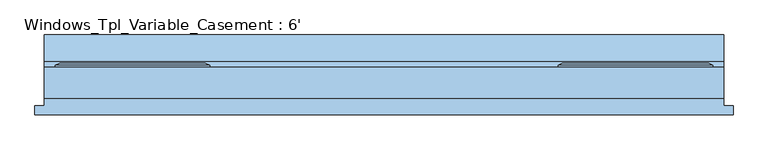
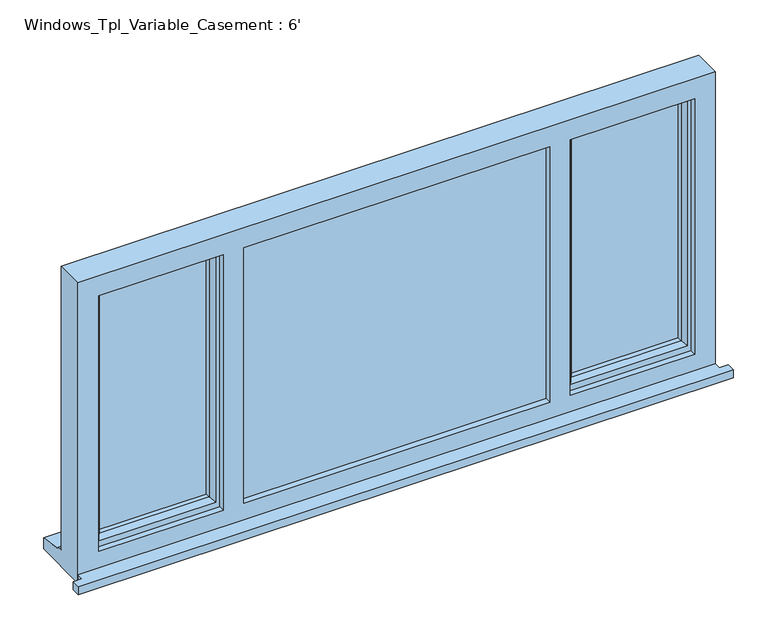
"""IFC4 building model written with IfcOpenShell, lengths in millimetres: window geometry, Windows_Tpl_Variable_Casement : 6'."""

from ifc_helpers import new_model, si_unit, frame, origin, place, context, project, spatial, polyline, outline, extrude, faceted_brep, source, transform, mapped, element, save


def windows_tpl_variable_casement_6_d811e495(model_context):
    return source(origin(), model_context, "Body", "SolidModel", [
        extrude(outline(polyline([(-1538.8, -92.7434322), (-1538.8, -67.7434322), (-1513.8, -67.7434322), (-1513.8, -48.3434322), (315.0, -48.3434322), (315.0, -67.7434322), (340.0, -67.7434322), (340.0, -92.7434322), (-1538.8, -92.7434322)])), frame((0.0, 0.0, 1200.0), z_axis=(0.0, 0.0, 1.0), x_axis=(1.0, 0.0, 0.0)), (0.0, 0.0, 1.0), 25.0),
        faceted_brep([(-130.0, 34.6565678, 2080.0), (-130.0, 40.4300705, 2080.0), (-130.0, 40.4300705, 1253.0), (-130.0, 34.6565678, 1253.0), (-120.0, -30.3434322, 2070.0), (-120.0, 34.6565678, 2070.0), (-120.0, 34.6565678, 1263.0), (-120.0, -30.3434322, 1263.0), (-80.0, -15.8505323, 2030.0), (-90.1480377, -30.3434322, 2040.1480377), (-90.1480377, -30.3434322, 1292.8519623), (-80.0, -15.8505323, 1303.0), (-80.0, -1.3434322, 2030.0), (-80.0, -1.3434322, 1303.0), (-90.0, 22.6565678, 2040.0), (-90.0, -1.3434322, 2040.0), (-90.0, -1.3434322, 1293.0), (-90.0, 22.6565678, 1293.0), (-80.0, 40.4300705, 2030.0), (-80.0, 22.6565678, 2030.0), (-80.0, 22.6565678, 1303.0), (-80.0, 40.4300705, 1303.0), (-97.4457548, 46.2035732, 2047.4457548), (-97.4457548, 46.2035732, 1285.5542452), (-119.2153903, 46.2035732, 2069.2153903), (-119.2153903, 46.2035732, 1263.7846097), (285.0, 40.4300705, 1253.0), (285.0, 34.6565678, 1253.0), (275.0, 34.6565678, 1263.0), (275.0, -30.3434322, 1263.0), (245.1480377, -30.3434322, 1292.8519623), (235.0, -15.8505323, 1303.0), (235.0, -1.3434322, 1303.0), (245.0, -1.3434322, 1293.0), (245.0, 22.6565678, 1293.0), (235.0, 22.6565678, 1303.0), (235.0, 40.4300705, 1303.0), (252.4457548, 46.2035732, 1285.5542452), (274.2153903, 46.2035732, 1263.7846097), (285.0, 40.4300705, 2080.0), (285.0, 34.6565678, 2080.0), (275.0, 34.6565678, 2070.0), (275.0, -30.3434322, 2070.0), (245.1480377, -30.3434322, 2040.1480377), (235.0, -15.8505323, 2030.0), (235.0, -1.3434322, 2030.0), (245.0, -1.3434322, 2040.0), (245.0, 22.6565678, 2040.0), (235.0, 22.6565678, 2030.0), (235.0, 40.4300705, 2030.0), (252.4457548, 46.2035732, 2047.4457548), (274.2153903, 46.2035732, 2069.2153903)], [[[0, 1, 2, 3]], [[4, 5, 6, 7]], [[8, 9, 10, 11]], [[12, 8, 11, 13]], [[14, 15, 16, 17]], [[18, 19, 20, 21]], [[22, 18, 21, 23]], [[1, 24, 25, 2]], [[3, 2, 26, 27]], [[7, 6, 28, 29]], [[11, 10, 30, 31]], [[13, 11, 31, 32]], [[17, 16, 33, 34]], [[21, 20, 35, 36]], [[23, 21, 36, 37]], [[2, 25, 38, 26]], [[27, 26, 39, 40]], [[29, 28, 41, 42]], [[31, 30, 43, 44]], [[32, 31, 44, 45]], [[34, 33, 46, 47]], [[36, 35, 48, 49]], [[37, 36, 49, 50]], [[26, 38, 51, 39]], [[40, 39, 1, 0]], [[3, 27, 40, 0], [5, 41, 28, 6]], [[42, 41, 5, 4]], [[7, 29, 42, 4], [9, 43, 30, 10]], [[44, 43, 9, 8]], [[45, 44, 8, 12]], [[15, 46, 33, 16], [13, 32, 45, 12]], [[47, 46, 15, 14]], [[17, 34, 47, 14], [19, 48, 35, 20]], [[49, 48, 19, 18]], [[50, 49, 18, 22]], [[24, 51, 38, 25], [23, 37, 50, 22]], [[39, 51, 24, 1]]]),
        faceted_brep([(-1068.8, 34.6565678, 2080.0), (-1068.8, 40.4300705, 2080.0), (-1483.8, 40.4300705, 2080.0), (-1483.8, 34.6565678, 2080.0), (-1078.8, -30.3434322, 2070.0), (-1078.8, 34.6565678, 2070.0), (-1473.8, 34.6565678, 2070.0), (-1473.8, -30.3434322, 2070.0), (-1118.8, -15.8505323, 2030.0), (-1108.6519623, -30.3434322, 2040.1480377), (-1443.9480377, -30.3434322, 2040.1480377), (-1433.8, -15.8505323, 2030.0), (-1118.8, -1.3434322, 2030.0), (-1433.8, -1.3434322, 2030.0), (-1108.8, 22.6565678, 2040.0), (-1108.8, -1.3434322, 2040.0), (-1443.8, -1.3434322, 2040.0), (-1443.8, 22.6565678, 2040.0), (-1118.8, 40.4300705, 2030.0), (-1118.8, 22.6565678, 2030.0), (-1433.8, 22.6565678, 2030.0), (-1433.8, 40.4300705, 2030.0), (-1099.9854344, 46.2035732, 2048.8145656), (-1452.6145656, 46.2035732, 2048.8145656), (-1080.4307806, 46.2035732, 2068.3692194), (-1472.1692194, 46.2035732, 2068.3692194), (-1483.8, 40.4300705, 1253.0), (-1483.8, 34.6565678, 1253.0), (-1473.8, 34.6565678, 1263.0), (-1473.8, -30.3434322, 1263.0), (-1443.9480377, -30.3434322, 1292.8519623), (-1433.8, -15.8505323, 1303.0), (-1433.8, -1.3434322, 1303.0), (-1443.8, -1.3434322, 1293.0), (-1443.8, 22.6565678, 1293.0), (-1433.8, 22.6565678, 1303.0), (-1433.8, 40.4300705, 1303.0), (-1452.6145656, 46.2035732, 1284.1854344), (-1472.1692194, 46.2035732, 1264.6307806), (-1068.8, 40.4300705, 1253.0), (-1068.8, 34.6565678, 1253.0), (-1078.8, 34.6565678, 1263.0), (-1078.8, -30.3434322, 1263.0), (-1108.6519623, -30.3434322, 1292.8519623), (-1118.8, -15.8505323, 1303.0), (-1118.8, -1.3434322, 1303.0), (-1108.8, -1.3434322, 1293.0), (-1108.8, 22.6565678, 1293.0), (-1118.8, 22.6565678, 1303.0), (-1118.8, 40.4300705, 1303.0), (-1099.9854344, 46.2035732, 1284.1854344), (-1080.4307806, 46.2035732, 1264.6307806)], [[[0, 1, 2, 3]], [[4, 5, 6, 7]], [[8, 9, 10, 11]], [[12, 8, 11, 13]], [[14, 15, 16, 17]], [[18, 19, 20, 21]], [[22, 18, 21, 23]], [[1, 24, 25, 2]], [[3, 2, 26, 27]], [[7, 6, 28, 29]], [[11, 10, 30, 31]], [[13, 11, 31, 32]], [[17, 16, 33, 34]], [[21, 20, 35, 36]], [[23, 21, 36, 37]], [[2, 25, 38, 26]], [[27, 26, 39, 40]], [[0, 3, 27, 40], [41, 28, 6, 5]], [[29, 28, 41, 42]], [[4, 7, 29, 42], [43, 30, 10, 9]], [[31, 30, 43, 44]], [[32, 31, 44, 45]], [[46, 33, 16, 15], [12, 13, 32, 45]], [[34, 33, 46, 47]], [[14, 17, 34, 47], [48, 35, 20, 19]], [[36, 35, 48, 49]], [[37, 36, 49, 50]], [[51, 38, 25, 24], [22, 23, 37, 50]], [[26, 38, 51, 39]], [[40, 39, 1, 0]], [[42, 41, 5, 4]], [[44, 43, 9, 8]], [[45, 44, 8, 12]], [[47, 46, 15, 14]], [[49, 48, 19, 18]], [[50, 49, 18, 22]], [[39, 51, 24, 1]]]),
        faceted_brep([(315.0, -48.3434322, 2110.0), (-1513.8, -48.3434322, 2110.0), (-1513.8, -48.3434322, 1200.0), (315.0, -48.3434322, 1200.0), (255.0, -48.3434322, 2050.0), (255.0, -48.3434322, 1275.0), (-102.0, -48.3434322, 1275.0), (-102.0, -48.3434322, 2050.0), (-160.0, -48.3434322, 2050.0), (-160.0, -48.3434322, 1275.0), (-1038.8, -48.3434322, 1275.0), (-1038.8, -48.3434322, 2050.0), (-1096.8, -48.3434322, 2050.0), (-1096.8, -48.3434322, 1275.0), (-1453.8, -48.3434322, 1275.0), (-1453.8, -48.3434322, 2050.0), (-1513.8, 34.6565678, 2110.0), (-1513.8, 34.6565678, 1251.0), (-1513.8, 49.6565678, 1249.68767), (-1513.8, 49.6565678, 1244.7449676), (-1513.8, 122.1565678, 1233.8088847), (-1513.8, 122.1565678, 1200.0), (315.0, 34.6565678, 2110.0), (315.0, 34.6565678, 1251.0), (-1473.8, 34.6565678, 2070.0), (-1473.8, 34.6565678, 1263.0), (-1078.8, 34.6565678, 1263.0), (-1078.8, 34.6565678, 2070.0), (-1038.8, 34.6565678, 2070.0), (-1038.8, 34.6565678, 1263.0), (-160.0, 34.6565678, 1263.0), (-160.0, 34.6565678, 2070.0), (-120.0, 34.6565678, 2070.0), (-120.0, 34.6565678, 1263.0), (275.0, 34.6565678, 1263.0), (275.0, 34.6565678, 2070.0), (-1473.8, -30.3434322, 2070.0), (-1473.8, -30.3434322, 1263.0), (-1048.8, -30.3434322, 2070.0), (-150.0, -30.3434322, 2070.0), (-150.0, -30.3434322, 1263.0), (-1048.8, -30.3434322, 1263.0), (-160.0, -30.3434322, 2050.0), (-1038.8, -30.3434322, 2050.0), (-1038.8, -30.3434322, 1275.0), (-160.0, -30.3434322, 1275.0), (-120.0, -30.3434322, 2070.0), (275.0, -30.3434322, 2070.0), (275.0, -30.3434322, 1263.0), (-120.0, -30.3434322, 1263.0), (255.0, -30.3434322, 2050.0), (-102.0, -30.3434322, 2050.0), (-102.0, -30.3434322, 1275.0), (255.0, -30.3434322, 1275.0), (-1078.8, -30.3434322, 2070.0), (-1078.8, -30.3434322, 1263.0), (-1096.8, -30.3434322, 2050.0), (-1453.8, -30.3434322, 2050.0), (-1453.8, -30.3434322, 1275.0), (-1096.8, -30.3434322, 1275.0), (-1038.8, -6.3434322, 2070.0), (-160.0, -6.3434322, 2070.0), (-150.0, -6.3434322, 2070.0), (-1048.8, -6.3434322, 2070.0), (315.0, 122.1565678, 1200.0), (315.0, 122.1565678, 1233.8088847), (315.0, 49.6565678, 1244.7449676), (315.0, 49.6565678, 1249.68767), (-1038.8, -6.3434322, 1263.0), (-1048.8, -6.3434322, 1263.0), (-150.0, -6.3434322, 1263.0), (-160.0, -6.3434322, 1263.0)], [[[0, 1, 2, 3], [4, 5, 6, 7], [8, 9, 10, 11], [12, 13, 14, 15]], [[2, 1, 16, 17, 18, 19, 20, 21]], [[17, 16, 22, 23], [24, 25, 26, 27], [28, 29, 30, 31], [32, 33, 34, 35]], [[25, 24, 36, 37]], [[38, 39, 40, 41], [42, 43, 44, 45]], [[46, 47, 48, 49], [50, 51, 52, 53]], [[36, 54, 55, 37], [56, 57, 58, 59]], [[57, 15, 14, 58]], [[1, 0, 22, 16]], [[36, 24, 27, 54]], [[35, 47, 46, 32]], [[60, 28, 31, 61, 62, 39, 38, 63]], [[15, 57, 56, 12]], [[50, 4, 7, 51]], [[11, 43, 42, 8]], [[23, 22, 0, 3, 64, 65, 66, 67]], [[35, 34, 48, 47]], [[4, 50, 53, 5]], [[43, 11, 10, 44]], [[12, 56, 59, 13]], [[27, 26, 55, 54]], [[29, 28, 60, 68]], [[68, 60, 63, 69]], [[69, 63, 38, 41]], [[62, 70, 40, 39]], [[70, 62, 61, 71]], [[71, 61, 31, 30]], [[33, 32, 46, 49]], [[51, 7, 6, 52]], [[8, 42, 45, 9]], [[64, 3, 2, 21]], [[65, 64, 21, 20]], [[66, 65, 20, 19]], [[67, 66, 19, 18]], [[23, 67, 18, 17]], [[26, 25, 37, 55]], [[34, 33, 49, 48]], [[41, 40, 70, 71, 30, 29, 68, 69]], [[6, 5, 53, 52]], [[45, 44, 10, 9]], [[59, 58, 14, 13]]]),
        extrude(outline(polyline([(-1108.8, -1.3434322), (-1443.8, -1.3434322), (-1443.8, 22.6565678), (-1108.8, 22.6565678), (-1108.8, -1.3434322)])), frame((0.0, 0.0, 1293.0), z_axis=(0.0, 0.0, 1.0), x_axis=(1.0, 0.0, 0.0)), (0.0, 0.0, 1.0), 747.0),
        extrude(outline(polyline([(-1048.8, -6.3434322), (-150.0, -6.3434322), (-150.0, -30.3434322), (-1048.8, -30.3434322), (-1048.8, -6.3434322)])), frame((0.0, 0.0, 1263.0), z_axis=(0.0, 0.0, 1.0), x_axis=(1.0, 0.0, 0.0)), (0.0, 0.0, 1.0), 807.0),
        extrude(outline(polyline([(245.0, -1.3434322), (-90.0, -1.3434322), (-90.0, 22.6565678), (245.0, 22.6565678), (245.0, -1.3434322)])), frame((0.0, 0.0, 1293.0), z_axis=(0.0, 0.0, 1.0), x_axis=(1.0, 0.0, 0.0)), (0.0, 0.0, 1.0), 747.0),
    ])


if __name__ == "__main__":
    model = new_model("IFC4")
    model_context = context("Model", 3, world=origin())
    ifc_project = project(units=[si_unit("LENGTHUNIT", "METRE", prefix="MILLI")], contexts=[model_context])
    site = spatial("IfcSite", under=ifc_project)
    building = spatial("IfcBuilding", under=site)
    placement = place(None, origin())
    windows_tpl_variable_casement_6_shape = windows_tpl_variable_casement_6_d811e495(model_context)
    element("IfcWindow", 1, ObjectType="Windows_Tpl_Variable_Casement : 6'", at=placement, inside=building, context=model_context, shape_type="MappedRepresentation", body=[
        mapped(windows_tpl_variable_casement_6_shape, transform((0.0, 0.0, 0.0), x_axis=(1.0, 0.0, 0.0), y_axis=(0.0, 1.0, 0.0), z_axis=(0.0, 0.0, 1.0))),
    ])
    save(model, "model.ifc")

# Revit data of these elements
# Type "Windows_Tpl_Variable_Casement : 6'"
#   Type Mark = "84"
#   Operation = "TriplePanelVertical"
#   Construction Type Id = "GSP4R"
#   Manufacturer = "Revit"
#   Keynote = "L10"
#   Analytic Construction = "1/8 in Pilkington single glazing"
#   Wrap Layers (Int) from Ext = 177.5 mm
#   Wrap Layers (Ext) from Ext = 102.5 mm
#   Window Board Projection = 25 mm
#   Window Board Extension = 25 mm
#   Visual Light Transmittance = 0.9
#   Solar Heat Gain Coefficient = 0.78
#   Rough Width = 1828.8 mm
#   Rough Height = 910 mm
#   Height = 910 mm
#   Width = 1828.8 mm
#   Heat Transfer Coefficient (U) = 3.6886 W/(m²·K)
#   Glazing Thickness = 24 mm
#   FrameOffset - External = 50 mm
#   Frame Depth = 65 mm
#   Default Head Height = 2110 mm
#   Cill Depth = 87.5 mm
#   Cavity Closer Width = 50 mm
#   Cavity Closer Offset from Ext = 102.5 mm
#   Cavity Closer Depth = 85 mm
#   Casement Width = 450 mm
#   Vis - Cavity Closers = yes
#   Define Thermal Properties by = 1
#   Material Trim = Window Frame
#   Material Glass = Glass
#   Material Frame = Window Frame
#   Wall Closure = (empty or 0)
# Element 1 (IfcWindow, "Windows_Tpl_Variable_Casement : 6'")
#   Materials on its faces: "Window Frame", "Glass"
# Materials
#   "Window Frame": colour RGB 249 249 249, transparency 0, Keynote = "L10", Cost = 0
#   "Glass": class "Glass", colour RGB 0 128 192, transparency 0.9, Description = "Soda Lime Glass", Cost = 0
